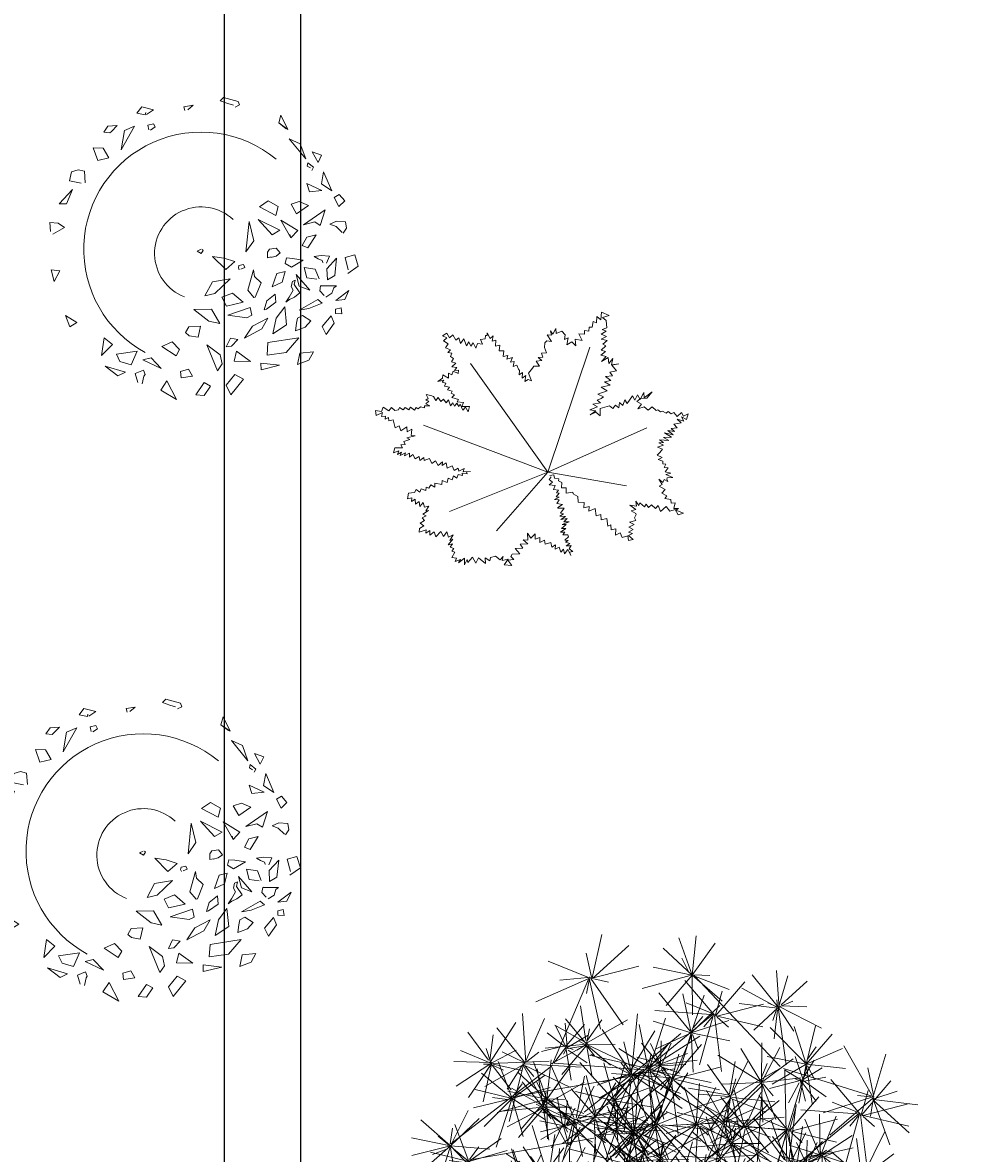
# Model space of a CAD drawing. Units: inches. Extents: x 8049 to 8459, y 820 to 1350.
# Tile 11 of 25: x 8132 to 8157, y 877 to 906. Entities that reach past the tile are written whole.
import ezdxf

# ---------------------------------------------------------------- set-up
doc = ezdxf.new("R2010")
doc.units = ezdxf.units.IN
doc.header["$MEASUREMENT"] = 0
doc.layers.add('A-ANNO-DIMS', color=2, linetype='Continuous', lineweight=18)
doc.layers.add('zelen', color=69, linetype='Continuous', lineweight=13)
doc.styles.get("Standard").update_dxf_attribs({"font": 'arial.ttf'})
doc.dimstyles.get("Standard").update_dxf_attribs({"dimtxt": 0.18, "dimasz": 0.18, "dimexe": 0.18, "dimexo": 0.0625, "dimgap": 0.09, "dimtad": 0, "dimtih": 1, "dimtoh": 1, "dimdec": 4, "dimzin": 0, "dimdsep": 46, "dimtxsty": 'Standard', "dimcen": 0.09, "dimadec": 0, "dimazin": 0, "dimtfac": 1, "dimtdec": 4, "dimtofl": 0, "dimtmove": 0, "dimatfit": 3, "dimfxl": 1, "dimtolj": 1, "dimtzin": 0, "dimarcsym": 0})

# ---------------------------------------------------------------- blocks, each defined once
blk = doc.blocks.new('z_96')
for p, q in [((-279.8, 149.9), (-254.2, 304.5)), ((-277.5, 143.8), (-209, 319.2)), ((-2.3, 183.5), (-55.4, 292.1)), ((0.6, 181.7), (29.5, 299.6)), ((-282.5, 143.4), (-440.4, 263.7)), ((-279.3, 139.9), (-326.8, 270.9)), ((1.7, 182.4), (-92.5, 262.1)), ((3.6, 188.7), (58.7, 265.3)), ((5.7, 184.9), (91.8, 284.8)), ((-276.5, 141.1), (-146.8, 221.3)), ((-9.6, 182.8), (-129.6, 222.9)), ((395.6, 94.6), (438.6, 246.5)), ((-292.1, 134.2), (-430.8, 180.4)), ((-5.7, 186.4), (-99.8, 114.3)), ((-4.6, 181.6), (-86.6, 72.3)), ((-0.6, 184.6), (125.7, 194.4)), ((1.5, 182.8), (69.9, 77.5)), ((9.8, 182.3), (88, 114.6)), ((393.4, 89.6), (354, 209.2)), ((393.4, 89.6), (479.1, 181.8)), ((-280.1, 150.3), (-304, 174)), ((-260.4, 142.3), (-97.9, 156.1)), ((-4.6, -3.2), (0.8, 176.4)), ((393.4, 89.6), (284.7, 153.1)), ((-283.2, 138.5), (-471.2, 114.9)), ((-279.1, 142.3), (-397.9, 16.9)), ((-285.6, 136.6), (-375, 92.2)), ((-277.6, 139.7), (-313.4, -1.1)), ((-279.1, 135.4), (-307.4, 99.5)), ((-278.4, 130.6), (-221.9, 40)), ((-277.5, 137.2), (-129.1, 19.3)), ((-17.8, -5.6), (-274.7, 141.8)), ((-263.2, 140.3), (-131, 113.5)), ((393.4, 89.6), (514.5, 123.6)), ((0, 0), (389.1, 84.4)), ((393.4, 89.6), (273.9, 50.1)), ((393.4, 89.6), (293.9, 12.5)), ((391.3, 83.5), (363.2, 41.9)), ((393.4, 89.6), (493.5, 13.4)), ((393.4, 89.6), (516.7, 64.5)), ((393.4, 89.6), (442.6, -26.2)), ((409.2, 93.4), (456.4, 89)), ((-74.7, -24.6), (-111.9, 37.5)), ((-71.7, -35.5), (-42.1, 65.4)), ((164.1, -89.9), (142.7, 11.7)), ((163.4, -89), (238.9, 7.6)), ((-237.5, -199.4), (-267, -22)), ((-10.4, -6), (-235.7, -205.3)), ((-74, -33), (-152.4, -40.5)), ((-65.2, -32.9), (-135.5, -11.4)), ((-76.2, -35.8), (-103.5, -105.8)), ((-80, -28.7), (-89.9, -20)), ((-16, -6.1), (-74.7, -37.4)), ((-72.5, -35.1), (-71.9, -112)), ((-68.1, -28.4), (-55.8, -19.3)), ((-5, -18.9), (163.8, -91.6)), ((159.3, -86.3), (85.5, -28.7)), ((167, -88.4), (276, -24.7)), ((-234, -202.3), (-196.3, -40.6)), ((-75, -39.2), (-157.1, -75.4)), ((-70.4, -41.1), (3.7, -57.1)), ((-69.9, -39.6), (-38.4, -102.6)), ((163.4, -86.5), (137.7, -55.7)), ((168.3, -88.4), (194, -71.5)), ((167.1, -94.6), (37.3, -175)), ((161.1, -92.4), (74, -95.2)), ((163.6, -101.8), (119, -170.9)), ((164.5, -93.4), (157.3, -141.4)), ((160.4, -93), (267.6, -148.2)), ((164.2, -92.2), (234.3, -170.2)), ((165.3, -92), (295.7, -74)), ((166.9, -90.5), (187.1, -100.1)), ((167, -104.1), (188, -212.9)), ((-237.4, -199.3), (-392.1, -169)), ((-246.4, -194), (-283.1, -163.8)), ((-231, -196), (-205.2, -161.9)), ((-242.3, -196.3), (-391.5, -241.3)), ((-242.2, -199.4), (-329.5, -310.3)), ((-241, -201.7), (-259.1, -277.3)), ((-242.2, -201.7), (-47.9, -207.3)), ((-236.2, -200.9), (-139.2, -306.8)), ((-230.8, -205.8), (-146.5, -236))]:
    blk.add_line(p, q)
blk = doc.blocks.new('сосна 1')
for p, rotation in [((317.7, 388.3), 121.1570021628385), ((-412.6, 386.5), 205.4822314301707), ((-117.1, 122.3), 55.05972244949475), ((-136.5, 361.1), 177.7388340989747), ((-351.5, 121.7), 257.3134436407499), ((285.8, 9.1), 60.73020616460848), ((-143.1, -5.5), 121.1570021628385), ((-343.1, -101.5), 57.88453704712605), ((234.4, -65.1), 73.8676290404427), ((-274, 161.3), 177.7388340989747), ((173.8, 17), 349.7944254651076), ((326.9, 45.9), 177.7388340989747), ((98.1, -4.6), 177.7388340989747), ((-502.4, -282.3), 279.7984529833926), ((-175.3, -367), 63.19571700542104), ((-48.9, -393.6), 342.5348703671633), ((260.9, -458.6), 13.72293452966709)]:
    blk.add_blockref('z_96', p, dxfattribs=dict(rotation=rotation))
blk = doc.blocks.new('z_85')
for p, q in [((168.5, 483.9), (169.7, 507.5)), ((169.7, 507.5), (194.7, 497.5)), ((140.4, 459.9), (144.1, 478.3)), ((144.1, 478.3), (154.8, 474.2)), ((154.8, 474.2), (155.6, 493.8)), ((155.6, 493.8), (168.5, 483.9)), ((194.7, 497.5), (173, 491.4)), ((173, 491.4), (185.2, 481.2)), ((185.2, 481.2), (186.9, 458.5)), ((-334.5, 433), (-320.5, 441.8)), ((-320.3, 426.3), (-334.5, 433)), ((-320.5, 441.8), (-312.2, 426.3)), ((-312.2, 426.3), (-302, 436.4)), ((-302, 436.4), (-292.5, 418.9)), ((-198.5, 423), (-198.2, 434.1)), ((-198.2, 434.1), (-192.6, 433.8)), ((-192.6, 433.8), (-192.5, 442.2)), ((-192.5, 442.2), (-183.3, 424.5)), ((-183.3, 424.5), (-173.3, 433.2)), ((-173.3, 433.2), (-176.4, 415.5)), ((-2.1, 435.8), (11.7, 434.9)), ((11.4, 414.5), (-2.1, 435.8)), ((8.4, 449), (15.4, 438)), ((11.7, 434.9), (8.4, 449)), ((15.4, 438), (25.6, 455.6)), ((25.6, 455.6), (26.4, 439.7)), ((26.4, 439.7), (44.1, 447.4)), ((44.1, 447.4), (54.4, 436.3)), ((54.4, 436.3), (52.3, 421.7)), ((98.5, 438.8), (116.6, 438)), ((108.9, 418.4), (98.5, 438.8)), ((116.1, 450.2), (130, 447.6)), ((116.6, 438), (116.1, 450.2)), ((130, 447.6), (130.9, 460.7)), ((130.9, 460.7), (140.4, 459.9)), ((185.1, 447.3), (169, 438)), ((169, 438), (186.4, 430.3)), ((186.9, 458.5), (172.1, 453.2)), ((172.1, 453.2), (185.1, 447.3)), ((-331, 417), (-320.3, 426.3)), ((-316.9, 407.2), (-331, 417)), ((-325.3, 394.5), (-316.9, 407.2)), ((-292.5, 418.9), (-282.7, 426.1)), ((-282.7, 426.1), (-277, 408.1)), ((-277, 408.1), (-266.3, 423.5)), ((-266.3, 423.5), (-258.7, 400.7)), ((-258.7, 400.7), (-250.8, 414.2)), ((-250.8, 414.2), (-244.9, 399.8)), ((-244.9, 399.8), (-237.2, 410.8)), ((-237.2, 410.8), (-228.5, 393.9)), ((-228.5, 393.9), (-223.5, 408.6)), ((-223.5, 408.6), (-207.8, 406.4)), ((-214.2, 421.3), (-198.5, 423)), ((-207.8, 406.4), (-214.2, 421.3)), ((-176.4, 415.5), (-165.1, 418.9)), ((-165.1, 418.9), (-166.4, 400.3)), ((-166.4, 400.3), (-152.4, 402.8)), ((-152.4, 402.8), (-154.8, 385.2)), ((-10.8, 396), (-9.6, 410.9)), ((-4.1, 379.1), (-10.8, 396)), ((-9.6, 410.9), (-3.8, 416.9)), ((-3.8, 416.9), (11.4, 414.5)), ((0, 0), (132.7, 397)), ((52.3, 421.7), (64.6, 426)), ((64.6, 426), (59.8, 403.9)), ((59.8, 403.9), (75.6, 414.2)), ((75.6, 414.2), (88.3, 401.4)), ((86.4, 422.5), (108.9, 418.4)), ((88.3, 401.4), (86.4, 422.5)), ((186.4, 430.3), (169.1, 422.7)), ((169.1, 422.7), (188.1, 417.5)), ((183.6, 400.7), (169.1, 387.1)), ((188.1, 417.5), (174.5, 406.5)), ((174.5, 406.5), (183.6, 400.7)), ((-309.5, 388.7), (-325.3, 394.5)), ((-317.2, 380.4), (-309.5, 388.7)), ((-305.1, 378.2), (-317.2, 380.4)), ((-309.5, 366.8), (-305.1, 378.2)), ((-299.2, 360.3), (-309.5, 366.8)), ((-305.9, 349.8), (-299.2, 360.3)), ((-154.8, 385.2), (-139.8, 385.6)), ((-139.8, 385.6), (-142, 367.5)), ((-142, 367.5), (-126.8, 370.7)), ((-126.8, 370.7), (-129.7, 358.9)), ((-129.7, 358.9), (-112.6, 364.1)), ((-112.6, 364.1), (-118.7, 349.7)), ((-31.2, 364.3), (-16.4, 364.7)), ((-19.6, 354.2), (-31.2, 364.3)), ((-19.9, 378.2), (-4.1, 379.1)), ((-16.4, 364.7), (-19.9, 378.2)), ((182.7, 383.5), (168.5, 371)), ((168.5, 371), (185.5, 367.5)), ((169.1, 387.1), (182.7, 383.5)), ((185.5, 367.5), (169.7, 351.3)), ((169.7, 351.3), (191.1, 364.1)), ((191.1, 364.1), (194, 345.3)), ((194, 345.3), (206.3, 360.8)), ((206.3, 360.8), (201.7, 341.2)), ((-292.6, 345.9), (-305.9, 349.8)), ((-305.3, 333.9), (-292.6, 345.9)), ((-288.9, 332.3), (-305.3, 333.9)), ((-296.8, 323.1), (-288.9, 332.3)), ((-283.1, 324), (-296.8, 323.1)), ((-284.3, 312.7), (-283.1, 324)), ((0, 0), (-245.8, 345.3)), ((-118.7, 349.7), (-106.5, 351.7)), ((-106.5, 351.7), (-110.4, 335.8)), ((-110.4, 335.8), (-98.6, 339.2)), ((-98.6, 339.2), (-92.9, 326.8)), ((-92.9, 326.8), (-89.6, 322.3)), ((-61.6, 314), (-48.8, 329.6)), ((-48.8, 329.6), (-45, 336.2)), ((-45, 336.2), (-26.1, 337)), ((-37.5, 352.7), (-19.6, 354.2)), ((-26.1, 337), (-37.5, 352.7)), ((201.7, 341.2), (224.8, 344.2)), ((224.8, 344.2), (203.2, 339.2)), ((203.2, 339.2), (217.5, 321.8)), ((-348.8, 287.5), (-334.3, 298.5)), ((-329.7, 291.9), (-348.8, 287.5)), ((-335.7, 285.2), (-329.7, 291.9)), ((-334.3, 298.5), (-333.4, 308.7)), ((-333.4, 308.7), (-315.2, 298.3)), ((-315.2, 298.3), (-314.9, 314.1)), ((-314.9, 314.1), (-305, 309.4)), ((-305, 309.4), (-300.9, 321)), ((-300.9, 321), (-284.3, 312.7)), ((-89.6, 322.3), (-91.1, 309)), ((-91.1, 309), (-80.4, 316.3)), ((-80.4, 316.3), (-81.2, 298.5)), ((-81.2, 298.5), (-70.2, 306.6)), ((-70.2, 306.6), (-73.6, 287.8)), ((-73.6, 287.8), (-62, 294.6)), ((-62, 294.6), (-51.7, 290.2)), ((-51.7, 290.2), (-61.6, 314)), ((199.8, 290.5), (179.5, 286.4)), ((204.7, 306.3), (183.1, 303.2)), ((183.1, 303.2), (199.8, 290.5)), ((217.5, 321.8), (196.8, 317.3)), ((196.8, 317.3), (204.7, 306.3)), ((-323.9, 282.5), (-335.7, 285.2)), ((-327.7, 273.4), (-323.9, 282.5)), ((-312.5, 269.8), (-327.7, 273.4)), ((-318.1, 260.9), (-312.5, 269.8)), ((-303.5, 257.1), (-318.1, 260.9)), ((-306.9, 250.2), (-303.5, 257.1)), ((187.9, 258.2), (158.6, 247.3)), ((198, 276.2), (169.3, 269.4)), ((169.3, 269.4), (187.9, 258.2)), ((179.5, 286.4), (198, 276.2)), ((292.5, 230.8), (304.2, 252.6)), ((304.2, 252.6), (305.4, 235.8)), ((305.4, 235.8), (330.6, 255.3)), ((330.6, 255.3), (314, 234.4)), ((-387.5, 216.4), (-377.3, 224.9)), ((-375.1, 210.9), (-387.5, 216.4)), ((-387.2, 228.2), (-380.3, 234.1)), ((-377.3, 224.9), (-387.2, 228.2)), ((-386.6, 246.8), (-370.9, 243.8)), ((-380.3, 234.1), (-386.6, 246.8)), ((-370.9, 243.8), (-362.5, 240.1)), ((-362.5, 240.1), (-355.4, 227.7)), ((-355.4, 227.7), (-347.7, 237.1)), ((-347.7, 237.1), (-340.1, 223.9)), ((-340.1, 223.9), (-331.2, 232.1)), ((-331.2, 232.1), (-323, 219.9)), ((-323, 219.9), (-314.9, 229.4)), ((-314.9, 229.4), (-308.7, 210.5)), ((-308.7, 210.5), (-301.4, 220.5)), ((-296.5, 245.4), (-306.9, 250.2)), ((-304.8, 236.9), (-296.5, 245.4)), ((-284, 230.8), (-304.8, 236.9)), ((-301.4, 220.5), (-296.2, 209.5)), ((-296.2, 209.5), (-288.7, 218.5)), ((-288.7, 218.5), (-282.8, 208)), ((-287.5, 222.7), (-284, 230.8)), ((-267.9, 221.3), (-287.5, 222.7)), ((-272.7, 208.1), (-267.9, 221.3)), ((166.6, 220), (142.5, 215.8)), ((142.5, 215.8), (157.5, 207.7)), ((169.1, 234), (156.5, 228.6)), ((156.5, 228.6), (166.6, 220)), ((158.6, 247.3), (176.5, 239.3)), ((176.5, 239.3), (169.1, 234)), ((225, 203.7), (227.4, 221.4)), ((227.4, 221.4), (237.6, 211.9)), ((237.6, 211.9), (244, 229.6)), ((244, 229.6), (251.2, 218.3)), ((251.2, 218.3), (269.1, 241.8)), ((269.1, 241.8), (276.1, 228.2)), ((276.1, 228.2), (284.6, 245.4)), ((291.9, 231.3), (282.8, 224.3)), ((282.8, 224.3), (297.7, 215.3)), ((284.6, 245.4), (292.5, 230.8)), ((294, 233.8), (291.9, 231.3)), ((314, 234.4), (294, 233.8)), ((-547.4, 195.4), (-527.9, 192.6)), ((-544.7, 179.5), (-547.4, 195.4)), ((-524.7, 189.5), (-544.7, 179.5)), ((-528.5, 176.6), (-524.7, 189.5)), ((-527.9, 192.6), (-523, 206.4)), ((-523, 206.4), (-504.7, 194.2)), ((-504.7, 194.2), (-496.5, 204.8)), ((-496.5, 204.8), (-486, 196.2)), ((-486, 196.2), (-473.8, 197.3)), ((-473.8, 197.3), (-470.6, 205)), ((-470.6, 205), (-459, 197.9)), ((-459, 197.9), (-453.2, 204.7)), ((-453.2, 204.7), (-441.7, 197.3)), ((-441.7, 197.3), (-436, 206.1)), ((-436, 206.1), (-423, 196.7)), ((-423, 196.7), (-417.9, 205.5)), ((-417.9, 205.5), (-411.3, 200.8)), ((-411.3, 200.8), (-403.9, 207.3)), ((-403.9, 207.3), (-392, 203.9)), ((-392, 203.9), (-391, 210.5)), ((-391, 210.5), (-375.1, 210.9)), ((-282.8, 208), (-278.3, 215.3)), ((-278.3, 215.3), (-269.6, 197)), ((-249.1, 208.6), (-272.7, 208.1)), ((-269.6, 197), (-261.6, 206.7)), ((-261.6, 206.7), (-252.6, 191.1)), ((-252.6, 191.1), (-249.1, 208.6)), ((157.5, 207.7), (133, 198.3)), ((133, 198.3), (152.7, 194.8)), ((152.7, 194.8), (134.2, 181.8)), ((134.2, 181.8), (152.3, 190.3)), ((152.3, 190.3), (165.5, 178.4)), ((165.5, 178.4), (166.1, 202.2)), ((166.1, 202.2), (195.8, 210)), ((195.8, 210), (206.3, 202.3)), ((206.3, 202.3), (214.9, 212.7)), ((214.9, 212.7), (225, 203.7)), ((297.7, 215.3), (285.2, 201.4)), ((285.2, 201.4), (305.7, 207.8)), ((305.7, 207.8), (318.4, 196.7)), ((318.4, 196.7), (331.5, 207.2)), ((331.5, 207.2), (343.4, 195.3)), ((343.4, 195.3), (349.2, 197.8)), ((349.2, 197.8), (357.1, 191.7)), ((357.1, 191.7), (363.4, 194)), ((363.4, 194), (375.4, 187.3)), ((375.4, 187.3), (381.6, 192.9)), ((381.6, 192.9), (391.6, 185.1)), ((391.6, 185.1), (399.5, 189.8)), ((399.5, 189.8), (410.7, 177.1)), ((410.7, 177.1), (423.8, 189)), ((423.8, 189), (430.9, 177.3)), ((430.9, 177.3), (445.2, 185.4)), ((445.2, 185.4), (440.2, 166.6)), ((-515.5, 177.6), (-528.5, 176.6)), ((-516.7, 167.9), (-515.5, 177.6)), ((-506.3, 173.2), (-516.7, 167.9)), ((-504.7, 162.4), (-506.3, 173.2)), ((-491.4, 165.7), (-504.7, 162.4)), ((-484.9, 140.6), (-491.4, 165.7)), ((-472, 147), (-484.9, 140.6)), ((-466.4, 131.1), (-472, 147)), ((-447.4, 143.9), (-466.4, 131.1)), ((-446.4, 127.5), (-447.4, 143.9)), ((0, 0), (-394.4, 149.4)), ((422.9, 156), (399.8, 152.7)), ((399.8, 152.7), (410.7, 140.5)), ((410.7, 167.7), (422.9, 156)), ((431.6, 161.5), (410.7, 167.7)), ((423.8, 175.6), (431.6, 161.5)), ((440.2, 166.6), (423.8, 175.6)), ((-447.3, 109), (-420.9, 115.7)), ((-437.9, 103.7), (-447.3, 109)), ((-431.2, 136.1), (-446.4, 127.5)), ((-433.6, 116.8), (-432.5, 124.7)), ((-420.9, 115.7), (-433.6, 116.8)), ((-432.5, 124.7), (-431.2, 136.1)), ((0, 0), (313.9, 140.8)), ((392.9, 111.3), (367, 110.4)), ((367, 110.4), (384, 100.5)), ((370, 124.5), (392.9, 111.3)), ((397.4, 117.9), (370, 124.5)), ((380.7, 131.9), (397.4, 117.9)), ((402.3, 129), (380.7, 131.9)), ((410.7, 140.5), (391.1, 138)), ((391.1, 138), (402.3, 129)), ((-490.1, 61.5), (-485.7, 76.6)), ((-485.7, 76.6), (-461.1, 77.2)), ((-466.3, 86.6), (-452.6, 88.2)), ((-461.1, 77.2), (-466.3, 86.6)), ((-456.8, 97.3), (-437.9, 103.7)), ((-452.6, 88.2), (-456.8, 97.3)), ((367.5, 85.5), (348.2, 79.7)), ((348.2, 79.7), (364, 72.5)), ((367.3, 93.6), (352.7, 93.5)), ((352.7, 93.5), (367.5, 85.5)), ((354.4, 102.3), (367.3, 93.6)), ((384, 100.5), (354.4, 102.3)), ((364, 72.5), (355.3, 62.8)), ((-472.7, 67.7), (-490.1, 61.5)), ((-477.3, 56.2), (-472.7, 67.7)), ((-464.1, 63.3), (-477.3, 56.2)), ((-468.4, 52.6), (-464.1, 63.3)), ((-452, 61.1), (-468.4, 52.6)), ((-455.1, 51.2), (-452, 61.1)), ((-439, 59.8), (-455.1, 51.2)), ((-439.5, 47.5), (-439, 59.8)), ((-428.5, 56.1), (-439.5, 47.5)), ((-421.5, 42.4), (-428.5, 56.1)), ((-408.4, 49.5), (-421.5, 42.4)), ((-406.6, 37.3), (-408.4, 49.5)), ((-393.5, 46.8), (-406.6, 37.3)), ((-392.2, 37), (-393.5, 46.8)), ((-375.3, 43.4), (-392.2, 37)), ((-368.7, 27.4), (-375.3, 43.4)), ((-356.3, 36.3), (-368.7, 27.4)), ((-348.5, 20.8), (-356.3, 36.3)), ((355.3, 62.8), (346.4, 53.6)), ((346.4, 53.6), (362.3, 46.4)), ((362.3, 46.4), (350.4, 40.1)), ((350.4, 40.1), (365.4, 35.2)), ((-333.9, 32.3), (-348.5, 20.8)), ((-335.5, 21.5), (-333.9, 32.3)), ((-322.4, 29.1), (-335.5, 21.5)), ((-319.9, 12.2), (-322.4, 29.1)), ((-303.8, 20), (-319.9, 12.2)), ((0, 0), (-312.2, -125)), ((-297.7, 5.3), (-303.8, 20)), ((-284.2, 12.8), (-297.7, 5.3)), ((-282.8, 2.5), (-284.2, 12.8)), ((-266.1, 11.6), (-282.8, 2.5)), ((-268.5, 0.9), (-266.1, 11.6)), ((-245.2, 1.9), (-268.5, 0.9)), ((-258.6, 1.3), (-245.2, 1.9)), ((-256.6, -5.5), (-258.6, 1.3)), ((0, 0), (-163.1, -186)), ((0, 0), (249.7, -43.2)), ((365.4, 35.2), (364.6, 26)), ((364.6, 26), (373.9, 25.2)), ((373.9, 25.2), (368.8, 14.6)), ((368.8, 14.6), (381.5, 13.5)), ((381.5, 13.5), (372.3, 1.1)), ((372.3, 1.1), (390.8, -3.1)), ((-358.6, -35.2), (-337, -39.8)), ((-358.3, -47.6), (-358.6, -35.2)), ((-337, -39.8), (-335.4, -26.5)), ((-335.4, -26.5), (-320, -32.7)), ((-320, -32.7), (-316.6, -19.6)), ((-316.6, -19.6), (-303.5, -24.4)), ((-303.5, -24.4), (-299.1, -12.1)), ((-299.1, -12.1), (-288.4, -18.9)), ((-288.4, -18.9), (-284.9, -7.8)), ((-284.9, -7.8), (-270.6, -10.5)), ((-272, -3.8), (-256.6, -5.5)), ((-270.6, -10.5), (-272, -3.8)), ((14.2, -31.5), (3.8, -40.4)), ((11, -15.5), (4.4, -23.3)), ((4.4, -23.3), (14.2, -31.5)), ((19.4, -9.1), (6, -11.1)), ((20.6, -19.7), (19.4, -9.1)), ((34.5, -21), (20.6, -19.7)), ((33.9, -27.7), (34.5, -21)), ((44.7, -33.5), (33.9, -27.7)), ((43.2, -50.4), (44.7, -33.5)), ((352.1, -22.6), (362.5, -39.2)), ((365.2, -32.7), (352.1, -22.6)), ((368.7, -23.2), (365.2, -32.7)), ((380.7, -30.1), (368.7, -23.2)), ((390.8, -3.1), (374.2, -7.2)), ((374.2, -7.2), (396.2, -16.9)), ((378.3, -17.7), (377.9, -21.9)), ((377.9, -21.9), (380.7, -30.1)), ((396.2, -16.9), (378.3, -17.7)), ((-445.6, -85.2), (-442.8, -66.9)), ((-442.8, -66.9), (-423.6, -64.7)), ((-423.6, -64.7), (-418.1, -55.3)), ((-418.1, -55.3), (-406.6, -63.9)), ((-406.6, -63.9), (-402.1, -52.8)), ((-402.1, -52.8), (-387.5, -58.3)), ((-387.5, -58.3), (-386, -47.3)), ((-386, -47.3), (-378.3, -50.6)), ((-378.3, -50.6), (-371.8, -40.4)), ((-371.8, -40.4), (-358.3, -47.6)), ((3.8, -40.4), (23.3, -42)), ((23.3, -42), (17.8, -55.3)), ((17.8, -55.3), (33.3, -57.2)), ((35.8, -67.3), (26.2, -78.5)), ((33.3, -57.2), (27.6, -66.1)), ((27.6, -66.1), (35.8, -67.3)), ((57.8, -49.8), (43.2, -50.4)), ((57.8, -66.7), (57.8, -49.8)), ((79.4, -63.3), (57.8, -66.7)), ((80.6, -68.6), (79.4, -63.3)), ((95, -77.7), (80.6, -68.6)), ((362.5, -39.2), (352.9, -44.5)), ((352.9, -44.5), (372.4, -54.8)), ((372.4, -54.8), (362.2, -67.3)), ((362.2, -67.3), (377.4, -74.9)), ((-431.8, -81.7), (-445.6, -85.2)), ((-433, -93.3), (-431.8, -81.7)), ((-421.5, -86.1), (-433, -93.3)), ((-420.3, -102.3), (-421.5, -86.1)), ((-408.9, -93.6), (-420.3, -102.3)), ((-406.5, -108.7), (-408.9, -93.6)), ((-396.2, -96.8), (-406.5, -108.7)), ((-391.4, -111), (-396.2, -96.8)), ((35.4, -79.2), (20.9, -86.9)), ((20.9, -86.9), (36.1, -88.5)), ((26.2, -78.5), (35.4, -79.2)), ((36.1, -88.5), (28.2, -99.3)), ((28.2, -99.3), (46.8, -102.9)), ((46.8, -102.9), (31.9, -112.9)), ((96.5, -95.7), (95, -77.7)), ((114.9, -96.9), (96.5, -95.7)), ((113.9, -113.2), (114.9, -96.9)), ((259.9, -104.5), (278.9, -118.5)), ((281.6, -108.4), (259.9, -104.5)), ((279.1, -92.7), (281.6, -108.4)), ((288.4, -105.6), (279.1, -92.7)), ((292.3, -97.7), (288.4, -105.6)), ((306.3, -109.8), (292.3, -97.7)), ((312.3, -101.9), (306.3, -109.8)), ((319.1, -112.6), (312.3, -101.9)), ((329.4, -104.1), (319.1, -112.6)), ((341.7, -115.9), (329.4, -104.1)), ((350.6, -106.3), (341.7, -115.9)), ((357.5, -125.6), (350.6, -106.3)), ((377.4, -74.9), (371.4, -84.3)), ((371.4, -84.3), (390.2, -87.1)), ((390.2, -87.1), (391, -98.7)), ((391, -98.7), (403.6, -97.7)), ((403.6, -97.7), (399.4, -115.7)), ((-399.4, -144.9), (-386, -138.6)), ((-396.7, -133.3), (-378.8, -121.8)), ((-386, -138.6), (-396.7, -133.3)), ((-377.3, -108.5), (-391.4, -111)), ((-387.6, -122.5), (-377.3, -108.5)), ((-378.8, -121.8), (-387.6, -122.5)), ((31.9, -112.9), (31.3, -114)), ((31.3, -114), (51.4, -114.8)), ((49.4, -132), (38, -139.7)), ((38, -139.7), (55.7, -140.9)), ((51.4, -114.8), (39.8, -130.3)), ((39.8, -130.3), (49.4, -132)), ((55.7, -140.9), (40.8, -150.5)), ((131.6, -109.3), (113.9, -113.2)), ((129.5, -124.2), (131.6, -109.3)), ((150, -116), (129.5, -124.2)), ((153.5, -138.6), (150, -116)), ((168.2, -134.7), (153.5, -138.6)), ((168.7, -151.1), (168.2, -134.7)), ((278.9, -118.5), (264.8, -122.8)), ((264.8, -122.8), (279.4, -131.9)), ((280.4, -134.4), (275.3, -145.6)), ((279.4, -131.9), (280.4, -134.4)), ((375.9, -109.5), (357.5, -125.6)), ((386.6, -123.9), (375.9, -109.5)), ((403.8, -118.5), (386.6, -123.9)), ((399.4, -115.7), (414.2, -115.6)), ((413.1, -135.8), (403.8, -118.5)), ((414.2, -115.6), (406.2, -120.7)), ((406.2, -120.7), (430, -130.9)), ((430, -130.9), (413.1, -135.8)), ((-408.7, -191.2), (-407.1, -178.7)), ((-407.1, -178.7), (-394, -170.7)), ((-405.7, -161.9), (-391.7, -153.5)), ((-394, -170.7), (-405.7, -161.9)), ((-391.7, -153.5), (-399.4, -144.9)), ((57.1, -178.7), (40.5, -191.1)), ((40.8, -150.5), (61.7, -147.7)), ((57.7, -166.9), (43.5, -179.6)), ((43.5, -179.6), (57.1, -178.7)), ((67.9, -157.4), (45.5, -166.6)), ((45.5, -166.6), (57.7, -166.9)), ((61.7, -147.7), (51.2, -158.2)), ((51.2, -158.2), (67.9, -157.4)), ((187.2, -147), (168.7, -151.1)), ((190.4, -171.9), (187.2, -147)), ((199.5, -167.6), (190.4, -171.9)), ((201.2, -183.5), (199.5, -167.6)), ((273.9, -166.2), (257.2, -175.1)), ((257.2, -175.1), (270.6, -182.1)), ((279.5, -153.9), (259.5, -159.1)), ((259.5, -159.1), (273.9, -166.2)), ((275.3, -145.6), (279.5, -153.9)), ((-386.3, -183.7), (-408.7, -191.2)), ((-386.9, -194.2), (-386.3, -183.7)), ((-375, -185.4), (-386.9, -194.2)), ((-374.4, -200.4), (-375, -185.4)), ((-361, -190), (-374.4, -200.4)), ((-355.6, -205.5), (-361, -190)), ((-340.1, -188.9), (-355.6, -205.5)), ((-331, -204.2), (-340.1, -188.9)), ((-320.5, -190.1), (-331, -204.2)), ((-315.8, -206.4), (-320.5, -190.1)), ((-316.4, -230.7), (-301.2, -212.5)), ((-300.9, -199.4), (-315.8, -206.4)), ((-311, -217.5), (-300.9, -199.4)), ((-301.2, -212.5), (-311, -217.5)), ((-78.5, -215.2), (-63.4, -228.2)), ((-63.1, -216.4), (-78.5, -215.2)), ((-64.5, -193.4), (-63.1, -216.4)), ((-54.1, -209.7), (-64.5, -193.4)), ((-39.9, -196.5), (-54.1, -209.7)), ((-40.4, -212.5), (-39.9, -196.5)), ((-25.3, -207.7), (-40.4, -212.5)), ((-25.3, -223.8), (-25.3, -207.7)), ((40.5, -191.1), (53.9, -190.4)), ((53.9, -190.4), (47.9, -199)), ((47.9, -199), (63.4, -198.7)), ((65.1, -205.6), (53.6, -216.1)), ((63.4, -198.7), (65.1, -205.6)), ((215.4, -180.2), (201.2, -183.5)), ((214.3, -200.6), (215.4, -180.2)), ((229.7, -192.5), (214.3, -200.6)), ((235.5, -207.5), (229.7, -192.5)), ((253.5, -202), (235.5, -207.5)), ((255.4, -217.1), (253.5, -202)), ((270.6, -214.1), (255.4, -217.1)), ((270.6, -182.1), (255.6, -190.7)), ((255.6, -190.7), (268.7, -194.5)), ((268.7, -194.5), (256, -201.4)), ((256, -201.4), (270.6, -214.1)), ((-303, -227.7), (-316.4, -230.7)), ((-309.9, -238.3), (-303, -227.7)), ((-298.3, -242.6), (-309.9, -238.3)), ((-304.7, -251.3), (-298.3, -242.6)), ((-295, -254.3), (-304.7, -251.3)), ((-79.8, -242), (-103.3, -242.6)), ((-103.3, -242.6), (-88.9, -260)), ((-63.4, -228.2), (-87.9, -229.1)), ((-87.9, -229.1), (-79.8, -242)), ((-10.7, -215.8), (-25.3, -223.8)), ((-8.3, -228.6), (-10.7, -215.8)), ((8.9, -223.5), (-8.3, -228.6)), ((12.7, -238.7), (8.9, -223.5)), ((24.7, -230.5), (12.7, -238.7)), ((23, -244.8), (24.7, -230.5)), ((35.5, -238.8), (23, -244.8)), ((40.7, -254.5), (35.5, -238.8)), ((49.8, -244.9), (40.7, -254.5)), ((52.7, -259.2), (49.8, -244.9)), ((63.6, -245.9), (52.7, -259.2)), ((53.6, -216.1), (64.9, -216.9)), ((64.9, -216.9), (56, -222.4)), ((56, -222.4), (69.4, -226.9)), ((69.4, -226.9), (58.1, -234.3)), ((58.1, -234.3), (70.9, -234.4)), ((72.4, -265), (63.6, -245.9)), ((73.9, -233.5), (67.9, -243.4)), ((67.9, -243.4), (79.4, -252.4)), ((70.9, -234.4), (73.9, -233.5)), ((-305.3, -270.9), (-295, -254.3)), ((-290.1, -273.1), (-305.3, -270.9)), ((-294.6, -284.2), (-290.1, -273.1)), ((-277.1, -277.7), (-294.6, -284.2)), ((-264.9, -273), (-283.1, -288.1)), ((-283.1, -288.1), (-277.1, -277.7)), ((-264.3, -294.3), (-264.9, -273)), ((-256.6, -277.5), (-264.3, -294.3)), ((-254.5, -286.6), (-256.6, -277.5)), ((-239.6, -270.1), (-254.5, -286.6)), ((-228.6, -289.1), (-239.6, -270.1)), ((-220, -272), (-228.6, -289.1)), ((-197.9, -289.9), (-220, -272)), ((-199.2, -272), (-197.9, -289.9)), ((-184.2, -282), (-199.2, -272)), ((-182.4, -271.4), (-184.2, -282)), ((-166.3, -266.5), (-182.4, -271.4)), ((-151.2, -278.6), (-166.3, -266.5)), ((-142.3, -267.5), (-151.2, -278.6)), ((-144.6, -280.3), (-142.3, -267.5)), ((-126.2, -276.2), (-144.6, -280.3)), ((-138.9, -294.9), (-126.2, -276.2)), ((-107.8, -278), (-127.3, -279.2)), ((-127.3, -279.2), (-114.3, -296.8)), ((-113.1, -261.1), (-117.3, -267.5)), ((-117.3, -267.5), (-107.8, -278)), ((-88.9, -260), (-113.1, -261.1)), ((79.4, -252.4), (68.2, -253.9)), ((68.2, -253.9), (72.4, -265)), ((-114.3, -296.8), (-138.9, -294.9))]:
    blk.add_line(p, q)
blk = doc.blocks.new('z_66')
for p, q in [((83.2, 488.9), (72.7, 477.7)), ((72.7, 477.7), (96.4, 469.7)), ((129.8, 476.2), (83.2, 488.9)), ((96.4, 469.7), (114.5, 463.9)), ((134, 464.6), (129.8, 476.2)), ((-176.4, 458.5), (-191.7, 438.6)), ((-191.7, 438.6), (-165.6, 433.5)), ((-139.2, 449.4), (-176.4, 458.5)), ((-165.6, 433.5), (-163.6, 441.1)), ((-165.6, 433.5), (-165.6, 433.5)), ((-161.1, 434.6), (-139.2, 449.4)), ((-13.6, 463.6), (-42.5, 459.2)), ((-42.5, 459.2), (-39.3, 446.9)), ((-30.3, 449.4), (-13.6, 463.6)), ((114.5, 463.9), (114.5, 463.9)), ((120.4, 457.8), (134, 464.6)), ((265.2, 432.1), (258.2, 407.5)), ((287.4, 387.2), (265.2, 432.1)), ((-283.6, 397.7), (-297.2, 378.2)), ((-254, 399.9), (-283.6, 397.7)), ((-272.8, 380.7), (-254, 399.9)), ((-241.9, 321.7), (-199.1, 397.3)), ((-199.1, 397.3), (-231.4, 383.6)), ((-138.9, 404.9), (-156.9, 400.2)), ((-156.9, 400.2), (-153.8, 385.4)), ((-133.3, 394.8), (-138.9, 404.9)), ((258.2, 407.5), (287.4, 387.2)), ((258.2, 407.5), (281.9, 388.6)), ((-297.2, 378.2), (-277.7, 376)), ((-277.7, 376), (-272.8, 380.7)), ((-231.4, 383.6), (-241.9, 321.7)), ((-148.6, 384.7), (-133.3, 394.8)), ((281.9, 388.6), (281.9, 388.6)), ((-330.3, 328.9), (-298.6, 327.1)), ((-316, 288.8), (-330.3, 328.9)), ((-298.6, 327.1), (-280.8, 297.1)), ((344.2, 293.1), (292, 357.2)), ((292, 357.2), (326.8, 341.2)), ((326.8, 341.2), (344.2, 293.1)), ((-280.8, 297.1), (-316, 288.8)), ((383.1, 281.9), (364.4, 316.3)), ((364.4, 316.3), (394.6, 305.1)), ((394.6, 305.1), (383.1, 281.9)), ((-399.2, 252.6), (-405.8, 224)), ((-377.9, 259.1), (-399.2, 252.6)), ((-358.4, 254), (-377.9, 259.1)), ((-356, 217.5), (-358.4, 254)), ((350.8, 280.8), (348.7, 270.3)), ((348.7, 270.3), (358.8, 264.5)), ((369.2, 266.7), (350.8, 280.8)), ((358.8, 264.5), (358.8, 264.5)), ((363.3, 256.6), (369.2, 266.7)), ((400.9, 251.9), (393.9, 214.6)), ((426.6, 192.2), (400.9, 251.9)), ((-405.8, 224), (-368.2, 216.4)), ((-368.2, 216.4), (-368.2, 216.4)), ((348, 215.7), (356, 188.9)), ((395.3, 193.2), (348, 215.7)), ((-396.4, 196.1), (-438.1, 150.2)), ((-414.8, 150.9), (-396.4, 196.1)), ((356, 188.9), (395.3, 193.2)), ((393.9, 214.6), (426.6, 192.2)), ((450, 180.6), (434.3, 171.2)), ((467.7, 160.3), (450, 180.6)), ((-438.1, 150.2), (-414.8, 150.9)), ((225.2, 159.9), (197, 140.8)), ((256.8, 142.6), (225.2, 159.9)), ((323.6, 157.8), (297.5, 149.8)), ((297.5, 149.8), (314.6, 119.4)), ((314.6, 119.4), (352.9, 145.5)), ((352.9, 145.5), (323.6, 157.8)), ((434.3, 171.2), (449.6, 142.6)), ((449.6, 142.6), (467.7, 160.3)), ((197, 140.8), (249.5, 113.6)), ((249.5, 113.6), (256.8, 142.6)), ((336.9, 84.3), (405.8, 131.7)), ((405.8, 131.7), (389.8, 82.1)), ((-468.4, 91.6), (-466.3, 62.6)), ((-441.6, 89), (-468.4, 91.6)), ((-458.3, 53.9), (-421.1, 76)), ((-421.1, 76), (-441.6, 89)), ((164.3, 94.8), (154.2, -2.2)), ((178.9, 33.3), (164.3, 94.8)), ((193.1, 101.3), (238, 52.1)), ((261.7, 66.6), (193.1, 101.3)), ((265.2, 98.8), (297.2, 42.7)), ((318.8, 66.2), (265.2, 98.8)), ((372.7, 93), (336.9, 84.3)), ((389.8, 82.1), (372.7, 93)), ((441.6, 95.9), (420.7, 86.5)), ((420.7, 86.5), (440.2, 78.5)), ((440.2, 78.5), (459.7, 59.7)), ((470.5, 93.7), (441.6, 95.9)), ((463.2, 57.9), (474, 73.5)), ((474, 73.5), (470.5, 93.7)), ((-466.3, 62.6), (-466.3, 62.6)), ((238, 52.1), (261.7, 66.6)), ((297.2, 42.7), (294.1, 53.6)), ((297.2, 42.7), (318.8, 66.2)), ((347.3, 45.2), (332.7, 18.1)), ((376.9, 52.5), (347.3, 45.2)), ((350.8, 10.9), (376.9, 52.5)), ((459.7, 59.7), (459.7, 59.7)), ((11.8, 6.2), (0, 0)), ((0, 0), (12.2, -6.9)), ((12.2, -6.9), (19.1, 2.9)), ((19.1, 2.9), (15.7, 5.8)), ((154.2, -2.2), (178.9, 33.3)), ((229, 7.2), (223.1, -2.5)), ((250.6, 9.8), (229, 7.2)), ((263.4, -5.4), (250.6, 9.8)), ((332.7, 18.1), (350.8, 10.9)), ((84.6, -21.7), (48, -17)), ((48, -17), (90.1, -58.3)), ((119.4, -32.9), (84.6, -21.7)), ((90.1, -58.3), (119.4, -32.9)), ((223.1, -2.5), (222.7, -20.6)), ((222.7, -20.6), (234.2, -18.1)), ((233.2, -19.9), (249.9, -15.9)), ((234.2, -18.1), (234.2, -18.1)), ((249.9, -15.9), (263.4, -5.4)), ((282.9, -21.3), (279.1, -39.1)), ((302.1, -22.8), (282.9, -21.3)), ((298.6, -50.3), (335.8, -28.6)), ((335.8, -28.6), (302.1, -22.8)), ((393.6, -13), (371, -17)), ((371, -17), (383.5, -23.5)), ((383.5, -23.5), (396.7, -28.9)), ((420, -15.9), (393.6, -13)), ((396.7, -28.9), (398.5, -35.5)), ((398.5, -35.5), (399.5, -35.8)), ((410.3, -38), (420, -15.9)), ((442, -22.4), (411.3, -55.4)), ((436, -77.1), (442, -22.4)), ((499.7, -10.9), (468.8, -19.9)), ((468.8, -19.9), (478.8, -58.6)), ((510.9, -47), (499.7, -10.9)), ((-464.2, -59.3), (-436.4, -62.6)), ((-454.5, -96.3), (-464.2, -59.3)), ((-436.4, -62.6), (-454.5, -96.3)), ((131.9, -44.9), (130.2, -52.5)), ((130.2, -52.5), (132.9, -59.3)), ((146.5, -42.3), (131.9, -44.9)), ((138.2, -56.8), (151, -51)), ((151, -51), (146.5, -42.3)), ((177.8, -59), (160.1, -123.8)), ((181, -80.3), (177.8, -59)), ((252.6, -70.9), (237.7, -112.9)), ((278.4, -64), (252.6, -70.9)), ((269.7, -98.4), (278.4, -64)), ((279.1, -39.1), (298.6, -50.3)), ((339, -51), (347.7, -84.3)), ((374.1, -56.8), (339, -51)), ((386.3, -87.9), (374.1, -56.8)), ((411.3, -55.4), (412.7, -90.8)), ((477.5, -70.2), (510.9, -47)), ((478.8, -58.6), (478.8, -58.6)), ((47.7, -96.6), (24, -141.9)), ((104.1, -87.9), (47.7, -96.6)), ((56, -133.9), (104.1, -87.9)), ((202.2, -100.6), (181, -80.3)), ((183.7, -145.5), (202.2, -100.6)), ((237.7, -112.9), (269.7, -98.4)), ((301.7, -95.5), (297.9, -112.2)), ((310.8, -91.9), (301.7, -95.5)), ((307.6, -106), (310.8, -91.9)), ((325.4, -132.4), (307.6, -106)), ((314.2, -74.2), (356.7, -123)), ((323.3, -111.1), (314.2, -74.2)), ((347.7, -84.3), (379.7, -88.3)), ((379.7, -88.3), (379.7, -88.3)), ((412.7, -90.8), (436, -77.1)), ((24, -141.9), (56, -133.9)), ((111.4, -132.8), (78.3, -146.2)), ((145.1, -162.1), (111.4, -132.8)), ((160.1, -123.8), (179.6, -146.6)), ((247.1, -135.7), (220.6, -157)), ((249.2, -162.1), (247.1, -135.7)), ((304.5, -123), (291.6, -145.8)), ((297.9, -112.2), (304.5, -123)), ((308.3, -145.8), (325.4, -132.4)), ((356.7, -123), (323.3, -111.1)), ((356.7, -123), (356.7, -123)), ((356.7, -123), (356.7, -123)), ((391.2, -110), (388.4, -125.6)), ((388.4, -125.6), (402.3, -140.8)), ((391.2, -110), (393.2, -108.6)), ((441.3, -110), (391.2, -110)), ((402.3, -140.8), (402.3, -140.8)), ((407.9, -145.5), (427, -133.5)), ((427, -133.5), (432.9, -115.8)), ((432.9, -115.8), (441.3, -110)), ((480.9, -124.5), (439.2, -156)), ((467.7, -153.4), (480.9, -124.5)), ((78.3, -146.2), (92.2, -174.1)), ((92.2, -174.1), (145.1, -162.1)), ((168.1, -178.4), (96.7, -202.6)), ((173, -203.4), (168.1, -178.4)), ((179.6, -146.6), (183.7, -145.5)), ((220.6, -157), (212.6, -186)), ((219.2, -183.5), (249.2, -162.1)), ((277.4, -176.2), (250.2, -212.4)), ((283.3, -233.8), (277.4, -176.2)), ((291.6, -145.8), (281.2, -161.8)), ((281.2, -161.8), (293, -152.7)), ((293, -152.7), (308.3, -145.8)), ((382.5, -152.7), (323.3, -187.4)), ((353.9, -182), (396.7, -164.3)), ((396.7, -164.3), (382.5, -152.7)), ((438.5, -183.8), (456.2, -179.1)), ((439.2, -156), (467.7, -153.4)), ((456.2, -179.1), (458.7, -199)), ((-417.9, -204.1), (-405.1, -239.6)), ((-382.8, -226.5), (-417.9, -204.1)), ((44.5, -184.2), (-10.8, -184.9)), ((-10.8, -184.9), (36.9, -222.2)), ((71, -229.1), (44.5, -184.2)), ((96.7, -202.6), (157.6, -211.3)), ((157.6, -211.3), (173, -203.4)), ((223.8, -212.4), (175.4, -237.7)), ((204.3, -246.8), (223.8, -212.4)), ((212.6, -186), (219.2, -183.5)), ((250.2, -212.4), (240.1, -262.4)), ((318.4, -212.1), (314.6, -228.7)), ((334.1, -203.7), (318.4, -212.1)), ((323.3, -187.4), (353.9, -182)), ((360.2, -221.1), (334.1, -203.7)), ((425.3, -204.5), (396.7, -238.5)), ((434.3, -228), (425.3, -204.5)), ((438.5, -197.6), (438.5, -183.8)), ((458.7, -199), (438.5, -197.6)), ((-405.1, -239.6), (-382.8, -226.5)), ((-26.4, -240.3), (-37.6, -258.4)), ((10.1, -237.7), (-26.4, -240.3)), ((2.4, -273.2), (10.1, -237.7)), ((36.9, -222.2), (71, -229.1)), ((175.4, -237.7), (149.6, -276.1)), ((149.6, -276.1), (204.3, -246.8)), ((240.1, -262.4), (283.3, -233.8)), ((314.6, -228.7), (311.8, -252.6)), ((311.8, -252.6), (320.5, -249.3)), ((320.5, -249.3), (342.8, -241.4)), ((342.8, -241.4), (360.2, -221.1)), ((396.7, -238.5), (409.2, -264.2)), ((409.2, -264.2), (434.3, -228)), ((-295.1, -275), (-304.2, -331.5)), ((-269, -296), (-295.1, -275)), ((-37.6, -258.4), (-25.8, -268.5)), ((-25.8, -268.5), (2.4, -273.2)), ((-25.8, -268.5), (-25.8, -268.5)), ((-25.8, -268.5), (-25.8, -268.5)), ((105.1, -276.1), (91.9, -303.6)), ((128.8, -280.4), (105.1, -276.1)), ((108.6, -301.4), (128.8, -280.4)), ((322.2, -275), (223.8, -290.2)), ((282.2, -321.7), (322.2, -275)), ((-304.2, -331.5), (-269, -296)), ((-191.1, -317.4), (-256.8, -326.4)), ((-209.8, -360.4), (-191.1, -317.4)), ((-80, -288), (-112.4, -302.5)), ((-112.4, -302.5), (-67.5, -331.8)), ((-56.7, -311.6), (-80, -288)), ((-67.5, -331.8), (-56.7, -311.6)), ((30.6, -297.1), (72.7, -329.3)), ((64, -379.6), (30.6, -297.1)), ((91.9, -303.6), (108.6, -301.4)), ((117.3, -348.8), (124.2, -317.7)), ((124.2, -317.7), (168.8, -349.9)), ((223.8, -290.2), (221.3, -330)), ((221.3, -330), (282.2, -321.7)), ((368.9, -319.2), (325.7, -323.9)), ((354.3, -346.3), (368.9, -319.2)), ((-256.8, -326.4), (-245.7, -350.3)), ((-245.7, -350.3), (-209.8, -360.4)), ((-172.6, -344.9), (-146.9, -338.7)), ((-114.8, -372.7), (-172.6, -344.9)), ((-146.9, -338.7), (-114.8, -372.7)), ((79.3, -357.9), (64, -379.6)), ((72.7, -329.3), (79.3, -357.9)), ((168.8, -349.9), (117.3, -348.8)), ((201.8, -355), (202.2, -376.3)), ((261, -362.2), (201.8, -355)), ((325.7, -323.9), (318.4, -360.1)), ((318.4, -360.1), (354.3, -346.3)), ((-292, -364.4), (-252, -395.5)), ((-228.3, -383.9), (-292, -364.4)), ((-252, -395.5), (-228.3, -383.9)), ((-197.3, -388.3), (-171.2, -377.8)), ((-188.3, -416.9), (-197.3, -388.3)), ((-171.2, -377.8), (-166, -391.5)), ((-166, -391.5), (-169.5, -396.6)), ((-27.8, -374.5), (-52.9, -381.8)), ((-52.9, -381.8), (-50.8, -402)), ((-15.3, -396.2), (-27.8, -374.5)), ((91.9, -424.8), (119, -391.5)), ((119, -391.5), (146.9, -406.4)), ((202.2, -376.3), (261, -362.2)), ((-169.5, -396.6), (-174.7, -420.5)), ((-174.7, -420.5), (-174.7, -420.5)), ((-116.2, -441.1), (-96.4, -411.8)), ((-96.4, -411.8), (-65.8, -470.8)), ((-50.8, -402), (-15.3, -396.2)), ((21.6, -417.2), (-4.5, -455.6)), ((42.1, -428.8), (21.6, -417.2)), ((21.6, -458.1), (42.1, -428.8)), ((106.8, -455.6), (91.9, -424.8)), ((146.9, -406.4), (106.8, -455.6)), ((-65.8, -470.8), (-116.2, -441.1)), ((-4.5, -455.6), (21.6, -458.1))]:
    blk.add_line(p, q)
for centre, radius, start, end in [((11.8, 6.2), 372.3, 50.2118, 241.5185), ((12.2, -6.9), 147.8, 46.7611, 248.9067)]:
    blk.add_arc(centre, radius, start, end)
blk = doc.blocks.new('*D58')
at = {"layer": 'A-ANNO-DIMS', "color": 0, "lineweight": -2, "transparency": 16777216}
for p, q in [((8139.397, 1162.808), (8139.397, 820.091)), ((8175.397, 1162.808), (8175.397, 820.091)), ((8139.577, 820.271), (8157.179, 820.271)), ((8175.217, 820.271), (8157.616, 820.271))]:
    blk.add_line(p, q, dxfattribs=at)
at = {"layer": 'A-ANNO-DIMS', "color": 0, "transparency": 16777216}
for points in [[(8139.577, 820.301), (8139.577, 820.241), (8139.397, 820.271)], [(8175.217, 820.301), (8175.217, 820.241), (8175.397, 820.271)]]:
    blk.add_solid(points, dxfattribs=at)
at = {"layer": 'Defpoints', "color": 0, "transparency": 16777216}
for p in [(8139.397, 1162.871), (8175.397, 1162.871), (8175.397, 820.271)]:
    blk.add_point(p, dxfattribs=at)
at = {"layer": 'A-ANNO-DIMS', "color": 0, "transparency": 16777216, "insert": (8157.397, 820.271), "char_height": 0.18, "attachment_point": 5}
blk.add_mtext('\\A1;36', dxfattribs=at)
blk = doc.blocks.new('*D70')
at = {"layer": 'A-ANNO-DIMS', "color": 0, "lineweight": -2, "transparency": 16777216}
for p, q in [((8083.397, 1045.808), (8083.397, 820.091)), ((8137.397, 1045.808), (8137.397, 820.091)), ((8083.577, 820.271), (8110.179, 820.271)), ((8137.217, 820.271), (8110.616, 820.271))]:
    blk.add_line(p, q, dxfattribs=at)
at = {"layer": 'A-ANNO-DIMS', "color": 0, "transparency": 16777216}
for points in [[(8083.577, 820.301), (8083.577, 820.241), (8083.397, 820.271)], [(8137.217, 820.301), (8137.217, 820.241), (8137.397, 820.271)]]:
    blk.add_solid(points, dxfattribs=at)
at = {"layer": 'Defpoints', "color": 0, "transparency": 16777216}
for p in [(8083.397, 1045.871), (8137.397, 1045.871), (8083.397, 820.271)]:
    blk.add_point(p, dxfattribs=at)
at = {"layer": 'A-ANNO-DIMS', "color": 0, "transparency": 16777216, "insert": (8110.397, 820.271), "char_height": 0.18, "attachment_point": 5}
blk.add_mtext('\\A1;54', dxfattribs=at)
blk = doc.blocks.new('*D76')
at = {"layer": 'A-ANNO-DIMS', "color": 0, "lineweight": -2, "transparency": 16777216}
for p, q in [((8083.397, 1054.808), (8083.397, 820.091)), ((8299.397, 1054.808), (8299.397, 820.091)), ((8083.577, 820.271), (8191.107, 820.271)), ((8299.217, 820.271), (8191.688, 820.271))]:
    blk.add_line(p, q, dxfattribs=at)
at = {"layer": 'A-ANNO-DIMS', "color": 0, "transparency": 16777216}
for points in [[(8083.577, 820.301), (8083.577, 820.241), (8083.397, 820.271)], [(8299.217, 820.301), (8299.217, 820.241), (8299.397, 820.271)]]:
    blk.add_solid(points, dxfattribs=at)
at = {"layer": 'Defpoints', "color": 0, "transparency": 16777216}
for p in [(8083.397, 1054.871), (8299.397, 1054.871), (8299.397, 820.271)]:
    blk.add_point(p, dxfattribs=at)
at = {"layer": 'A-ANNO-DIMS', "color": 0, "transparency": 16777216, "insert": (8191.397, 820.271), "char_height": 0.18, "attachment_point": 5}
blk.add_mtext('\\A1;216', dxfattribs=at)
blk = doc.blocks.new('*D88')
at = {"layer": 'A-ANNO-DIMS', "color": 0, "lineweight": -2, "transparency": 16777216}
for p, q in [((8083.397, 1162.808), (8083.397, 820.091)), ((8139.397, 1162.808), (8139.397, 820.091)), ((8083.577, 820.271), (8111.179, 820.271)), ((8139.217, 820.271), (8111.616, 820.271))]:
    blk.add_line(p, q, dxfattribs=at)
at = {"layer": 'A-ANNO-DIMS', "color": 0, "transparency": 16777216}
for points in [[(8083.577, 820.301), (8083.577, 820.241), (8083.397, 820.271)], [(8139.217, 820.301), (8139.217, 820.241), (8139.397, 820.271)]]:
    blk.add_solid(points, dxfattribs=at)
at = {"layer": 'Defpoints', "color": 0, "transparency": 16777216}
for p in [(8083.397, 1162.871), (8139.397, 1162.871), (8139.397, 820.271)]:
    blk.add_point(p, dxfattribs=at)
at = {"layer": 'A-ANNO-DIMS', "color": 0, "transparency": 16777216, "insert": (8111.397, 820.271), "char_height": 0.18, "attachment_point": 5}
blk.add_mtext('\\A1;56', dxfattribs=at)

msp = doc.modelspace()

# ---------------------------------------------------------------- block references
at = {"layer": 'zelen', "xscale": 0.0082668533249786, "yscale": 0.0082668533249786, "zscale": 0.0082668533249786}
for name, p in [('z_66', (8136.6914, 900.2752)), ('z_85', (8145.8888, 894.4772)), ('z_66', (8135.1758, 884.4775)), ('сосна 1', (8149.3607, 875.6575))]:
    msp.add_blockref(name, p, dxfattribs=at)

# ---------------------------------------------------------------- dimensions: what is measured, and where the dimension line sits
at = {"layer": 'A-ANNO-DIMS'}
for base, p1, p2, picture, middle in [((8139.3974, 820.2706), (8083.3974, 1162.8706), (8139.3974, 1162.8706), '*D88', (8111.3974, 820.2706)), ((8175.3974, 820.2706), (8139.3974, 1162.8706), (8175.3974, 1162.8706), '*D58', (8157.3974, 820.2706)), ((8299.3974, 820.2706), (8083.3974, 1054.8706), (8299.3974, 1054.8706), '*D76', (8191.3974, 820.2706)), ((8083.3974, 820.2706), (8137.3974, 1045.8706), (8083.3974, 1045.8706), '*D70', (8110.3974, 820.2706))]:
    dim = msp.add_linear_dim(base=base, p1=p1, p2=p2, dimstyle='Standard', override={"dimdec": 0, "dimlfac": 1, "dimrnd": 0, "dimzin": 0, "dimdsep": 46, "dimlunit": 2}, dxfattribs=at)
    dim.commit()
    dim.dimension.update_dxf_attribs({"geometry": picture, "text_midpoint": middle})

doc.saveas('drawing.dxf')
